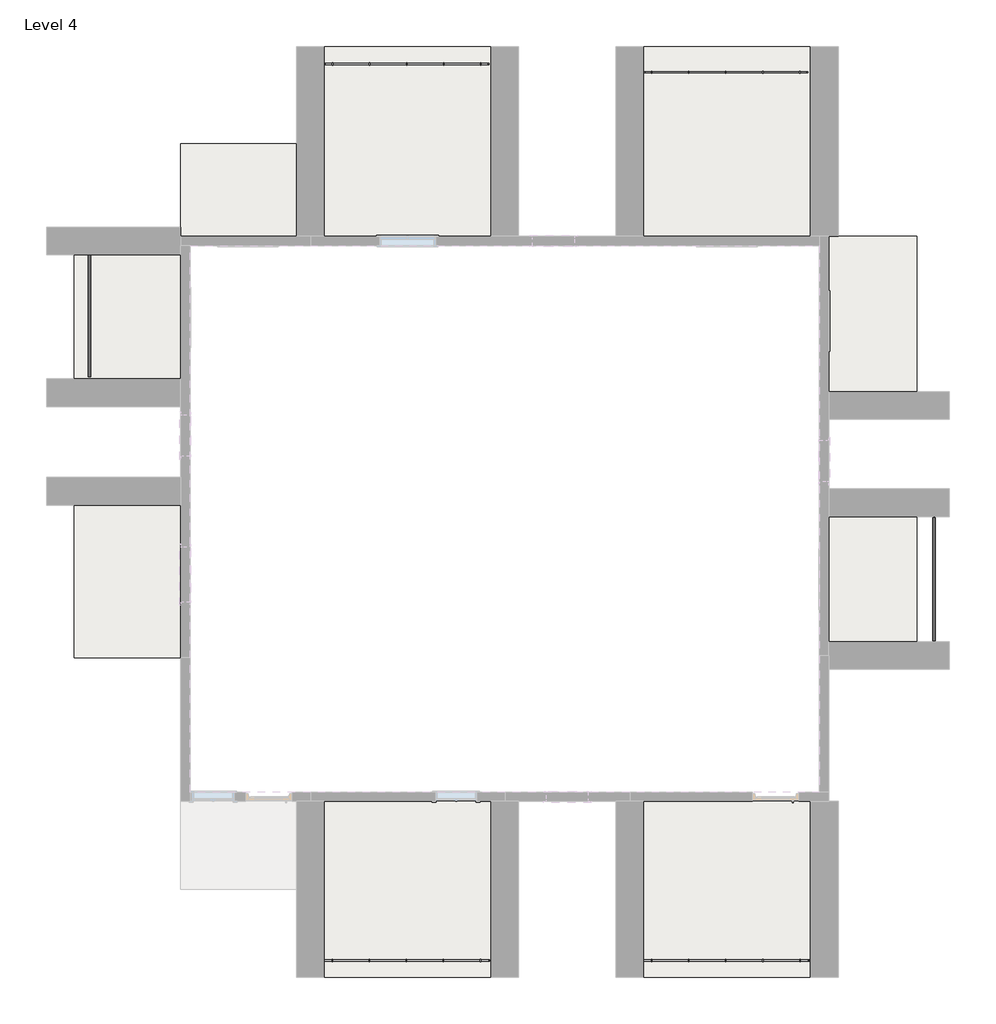
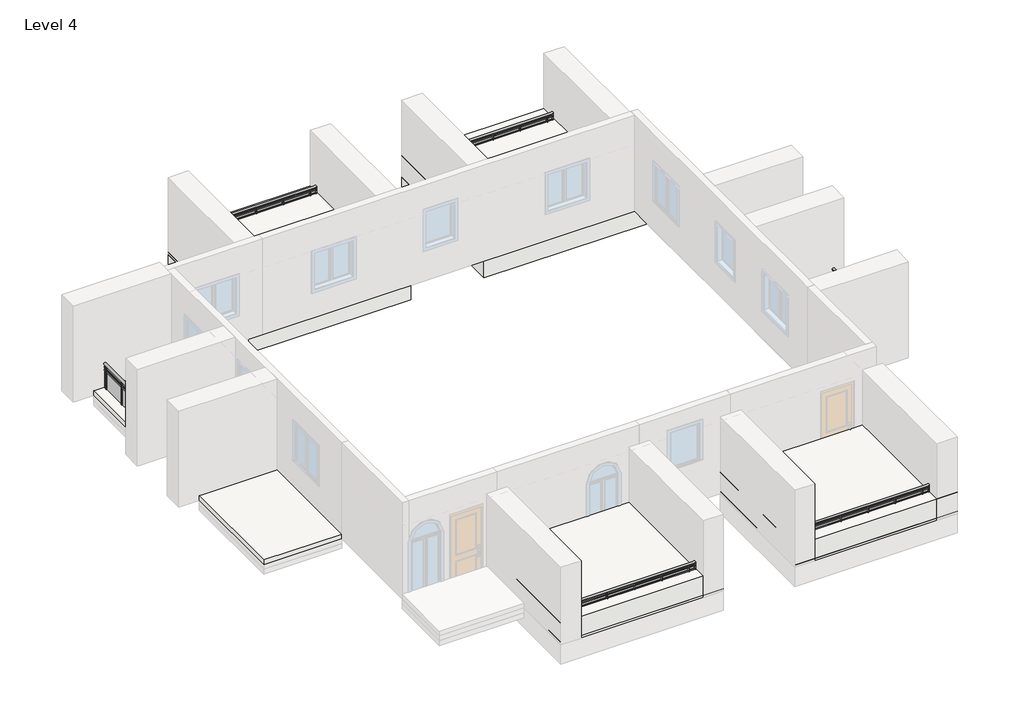
# One storey, part 2 of 2: 6 railings, 5 slabs.
"""IFC4 building model written with IfcOpenShell, lengths in millimetres."""

from ifc_helpers import new_model, si_unit, point, frame, origin, place, context, project, spatial, polyline, ellipse_curve, trimmed, outline, extrude, element, save
from ifc_brep_helpers import plane_surface, extruded_surface, advanced_brep

model = new_model("IFC4")

# Units and contexts
model_context = context("Model", 3, world=origin())
ifc_project = project(units=[si_unit("LENGTHUNIT", "METRE", prefix="MILLI")], contexts=[model_context])

# Site, building, storey
site = spatial("IfcSite", under=ifc_project)
building = spatial("IfcBuilding", under=site)
storey = spatial("IfcBuildingStorey", under=building, Name="Level 4", Elevation=9144.0)

# Railings
placement = place(None, origin())
element("IfcRailing", 1, ObjectType="Glass Panel - Bottom Fill", at=placement, inside=storey, context=model_context, shape_type="SolidModel", body=[
    advanced_brep(
    [(-9258.4937431, -9324.2034265, 10363.2), (-9258.4937431, -9400.4034265, 10363.2), (-5600.8937431, -9324.2034265, 10363.2), (-5600.8937431, -9400.4034265, 10363.2)],
    [
        (0, 1, ellipse_curve(frame((-9258.4937431, -9362.3034265, 10363.2), z_axis=(-1.0, 0.0, 0.0), x_axis=(0.0, -1.0, 0.0)), 38.1, 28.575)),
        (1, 0, ellipse_curve(frame((-9258.4937431, -9362.3034265, 10363.2), z_axis=(-1.0, 0.0, 0.0), x_axis=(0.0, -1.0, 0.0)), 38.1, 28.575)),
        (2, 3, ellipse_curve(frame((-5600.8937431, -9362.3034265, 10363.2), z_axis=(1.0, 0.0, 0.0), x_axis=(0.0, -1.0, 0.0)), 38.1, 28.575)),
        (3, 2, ellipse_curve(frame((-5600.8937431, -9362.3034265, 10363.2), z_axis=(1.0, 0.0, 0.0), x_axis=(0.0, -1.0, 0.0)), 38.1, 28.575)),
        (0, 2),
        (3, 1),
    ],
    [
        plane_surface(frame((-9258.4937431, -9362.3034265, 10363.2), z_axis=(-1.0, 0.0, 0.0), x_axis=(0.0, 1.0, 0.0))),
        plane_surface(frame((-5600.8937431, -9362.3034265, 10363.2), z_axis=(1.0, 0.0, 0.0), x_axis=(0.0, 1.0, 0.0))),
        extruded_surface(trimmed(ellipse_curve(frame((-5600.8937431, -9362.3034265, 10363.2), z_axis=(-1.0, 0.0, 0.0), x_axis=(0.0, -1.0, 0.0)), 38.1, 28.575), [point((-5600.8937431, -9324.2034265, 10363.2))], [point((-5600.8937431, -9400.4034265, 10363.2))], True, "CARTESIAN"), (-3657.5999999999995, 0.0, 0.0), 3657.5999999999995),
        extruded_surface(trimmed(ellipse_curve(frame((-5600.8937431, -9362.3034265, 10363.2), z_axis=(-1.0, 0.0, 0.0), x_axis=(0.0, -1.0, 0.0)), 38.1, 28.575), [point((-5600.8937431, -9400.4034265, 10363.2))], [point((-5600.8937431, -9324.2034265, 10363.2))], True, "CARTESIAN"), (-3657.5999999999995, 0.0, 0.0), 3657.5999999999995),
    ],
    [
        (0, [[1, 2]]),
        (1, [[3, 4]]),
        (2, [[-1, 5, -4, 6]]),
        (3, [[-2, -6, -3, -5]]),
    ],
),
    extrude(outline(polyline([(-9258.4937431, -9375.0034265), (-9258.4937431, -9349.6034265), (-5600.8937431, -9349.6034265), (-5600.8937431, -9375.0034265), (-9258.4937431, -9375.0034265)])), frame((0.0, 0.0, 10248.9), z_axis=(0.0, 0.0, 1.0), x_axis=(1.0, 0.0, 0.0)), (0.0, 0.0, 1.0), 25.4),
    extrude(outline(polyline([(-9258.4937431, -9375.0034265), (-9258.4937431, -9349.6034265), (-5600.8937431, -9349.6034265), (-5600.8937431, -9375.0034265), (-9258.4937431, -9375.0034265)])), frame((0.0, 0.0, 10147.3), z_axis=(0.0, 0.0, 1.0), x_axis=(1.0, 0.0, 0.0)), (0.0, 0.0, 1.0), 25.4),
    extrude(outline(polyline([(-5810.4437431, -9387.7034265), (-5810.4437431, -9336.9034265), (-5797.7437431, -9336.9034265), (-5797.7437431, -9387.7034265), (-5810.4437431, -9387.7034265)])), frame((0.0, 0.0, 9448.8), z_axis=(0.0, 0.0, 1.0), x_axis=(1.0, 0.0, 0.0)), (0.0, 0.0, 1.0), 885.6788223),
    extrude(outline(polyline([(-6616.8937431, -9355.7682695), (-5804.0937431, -9355.7682695), (-5804.0937431, -9362.1182695), (-6616.8937431, -9362.1182695), (-6616.8937431, -9355.7682695)])), frame((0.0, 0.0, 9550.4), z_axis=(0.0, 0.0, 1.0), x_axis=(1.0, 0.0, 0.0)), (0.0, 0.0, 1.0), 596.9),
    extrude(outline(polyline([(-6623.2437431, -9387.7034265), (-6623.2437431, -9336.9034265), (-6610.5437431, -9336.9034265), (-6610.5437431, -9387.7034265), (-6623.2437431, -9387.7034265)])), frame((0.0, 0.0, 9448.8), z_axis=(0.0, 0.0, 1.0), x_axis=(1.0, 0.0, 0.0)), (0.0, 0.0, 1.0), 885.6788223),
    extrude(outline(polyline([(-7429.6937431, -9355.7682695), (-6616.8937431, -9355.7682695), (-6616.8937431, -9362.1182695), (-7429.6937431, -9362.1182695), (-7429.6937431, -9355.7682695)])), frame((0.0, 0.0, 9550.4), z_axis=(0.0, 0.0, 1.0), x_axis=(1.0, 0.0, 0.0)), (0.0, 0.0, 1.0), 596.9),
    extrude(outline(polyline([(-7436.0437431, -9387.7034265), (-7436.0437431, -9336.9034265), (-7423.3437431, -9336.9034265), (-7423.3437431, -9387.7034265), (-7436.0437431, -9387.7034265)])), frame((0.0, 0.0, 9448.8), z_axis=(0.0, 0.0, 1.0), x_axis=(1.0, 0.0, 0.0)), (0.0, 0.0, 1.0), 885.6788223),
    extrude(outline(polyline([(-8242.4937431, -9355.7682695), (-7429.6937431, -9355.7682695), (-7429.6937431, -9362.1182695), (-8242.4937431, -9362.1182695), (-8242.4937431, -9355.7682695)])), frame((0.0, 0.0, 9550.4), z_axis=(0.0, 0.0, 1.0), x_axis=(1.0, 0.0, 0.0)), (0.0, 0.0, 1.0), 596.9),
    extrude(outline(polyline([(-8248.8437431, -9387.7034265), (-8248.8437431, -9336.9034265), (-8236.1437431, -9336.9034265), (-8236.1437431, -9387.7034265), (-8248.8437431, -9387.7034265)])), frame((0.0, 0.0, 9448.8), z_axis=(0.0, 0.0, 1.0), x_axis=(1.0, 0.0, 0.0)), (0.0, 0.0, 1.0), 885.6788223),
    extrude(outline(polyline([(-9055.2937431, -9355.7682695), (-8242.4937431, -9355.7682695), (-8242.4937431, -9362.1182695), (-9055.2937431, -9362.1182695), (-9055.2937431, -9355.7682695)])), frame((0.0, 0.0, 9550.4), z_axis=(0.0, 0.0, 1.0), x_axis=(1.0, 0.0, 0.0)), (0.0, 0.0, 1.0), 596.9),
    extrude(outline(polyline([(-9061.6437431, -9387.7034265), (-9061.6437431, -9336.9034265), (-9048.9437431, -9336.9034265), (-9048.9437431, -9387.7034265), (-9061.6437431, -9387.7034265)])), frame((0.0, 0.0, 9448.8), z_axis=(0.0, 0.0, 1.0), x_axis=(1.0, 0.0, 0.0)), (0.0, 0.0, 1.0), 885.6788223),
    extrude(outline(polyline([(-5613.5937431, -9371.8284265), (-5613.5937431, -9352.7784265), (-5594.5437431, -9352.7784265), (-5594.5437431, -9371.8284265), (-5613.5937431, -9371.8284265)])), frame((0.0, 0.0, 9448.8), z_axis=(0.0, 0.0, 1.0), x_axis=(1.0, 0.0, 0.0)), (0.0, 0.0, 1.0), 885.6788223),
    extrude(outline(polyline([(-9264.8437431, -9371.8284265), (-9264.8437431, -9352.7784265), (-9245.7937431, -9352.7784265), (-9245.7937431, -9371.8284265), (-9264.8437431, -9371.8284265)])), frame((0.0, 0.0, 9448.8), z_axis=(0.0, 0.0, 1.0), x_axis=(1.0, 0.0, 0.0)), (0.0, 0.0, 1.0), 885.6788223),
])
element("IfcRailing", 2, ObjectType="Glass Panel - Bottom Fill", at=placement, inside=storey, context=model_context, shape_type="SolidModel", body=[
    advanced_brep(
    [(-2248.0325613, -9324.2034265, 10358.1393423), (-2248.0325613, -9400.4034265, 10358.1393423), (1409.5674387, -9324.2034265, 10358.1393423), (1409.5674387, -9400.4034265, 10358.1393423)],
    [
        (0, 1, ellipse_curve(frame((-2248.0325613, -9362.3034265, 10358.1393423), z_axis=(-1.0, 0.0, 0.0), x_axis=(0.0, -1.0, 0.0)), 38.1, 28.575)),
        (1, 0, ellipse_curve(frame((-2248.0325613, -9362.3034265, 10358.1393423), z_axis=(-1.0, 0.0, 0.0), x_axis=(0.0, -1.0, 0.0)), 38.1, 28.575)),
        (2, 3, ellipse_curve(frame((1409.5674387, -9362.3034265, 10358.1393423), z_axis=(1.0, 0.0, 0.0), x_axis=(0.0, -1.0, 0.0)), 38.1, 28.575)),
        (3, 2, ellipse_curve(frame((1409.5674387, -9362.3034265, 10358.1393423), z_axis=(1.0, 0.0, 0.0), x_axis=(0.0, -1.0, 0.0)), 38.1, 28.575)),
        (0, 2),
        (3, 1),
    ],
    [
        plane_surface(frame((-2248.0325613, -9362.3034265, 10358.1393423), z_axis=(-1.0, 0.0, 0.0), x_axis=(0.0, 1.0, 0.0))),
        plane_surface(frame((1409.5674387, -9362.3034265, 10358.1393423), z_axis=(1.0, 0.0, 0.0), x_axis=(0.0, 1.0, 0.0))),
        extruded_surface(trimmed(ellipse_curve(frame((1409.5674387, -9362.3034265, 10358.1393423), z_axis=(-1.0, 0.0, 0.0), x_axis=(0.0, -1.0, 0.0)), 38.1, 28.575), [point((1409.5674387, -9324.2034265, 10358.1393423))], [point((1409.5674387, -9400.4034265, 10358.1393423))], True, "CARTESIAN"), (-3657.6, 0.0, 0.0), 3657.6),
        extruded_surface(trimmed(ellipse_curve(frame((1409.5674387, -9362.3034265, 10358.1393423), z_axis=(-1.0, 0.0, 0.0), x_axis=(0.0, -1.0, 0.0)), 38.1, 28.575), [point((1409.5674387, -9400.4034265, 10358.1393423))], [point((1409.5674387, -9324.2034265, 10358.1393423))], True, "CARTESIAN"), (-3657.6, 0.0, 0.0), 3657.6),
    ],
    [
        (0, [[1, 2]]),
        (1, [[3, 4]]),
        (2, [[-1, 5, -4, 6]]),
        (3, [[-2, -6, -3, -5]]),
    ],
),
    extrude(outline(polyline([(-2248.0325613, -9375.0034265), (-2248.0325613, -9349.6034265), (1409.5674387, -9349.6034265), (1409.5674387, -9375.0034265), (-2248.0325613, -9375.0034265)])), frame((0.0, 0.0, 10243.8393423), z_axis=(0.0, 0.0, 1.0), x_axis=(1.0, 0.0, 0.0)), (0.0, 0.0, 1.0), 25.4),
    extrude(outline(polyline([(-2248.0325613, -9375.0034265), (-2248.0325613, -9349.6034265), (1409.5674387, -9349.6034265), (1409.5674387, -9375.0034265), (-2248.0325613, -9375.0034265)])), frame((0.0, 0.0, 10142.2393423), z_axis=(0.0, 0.0, 1.0), x_axis=(1.0, 0.0, 0.0)), (0.0, 0.0, 1.0), 25.4),
    extrude(outline(polyline([(1200.0174387, -9387.7034265), (1200.0174387, -9336.9034265), (1212.7174387, -9336.9034265), (1212.7174387, -9387.7034265), (1200.0174387, -9387.7034265)])), frame((0.0, 0.0, 9443.7393423), z_axis=(0.0, 0.0, 1.0), x_axis=(1.0, 0.0, 0.0)), (0.0, 0.0, 1.0), 885.6788223),
    extrude(outline(polyline([(393.5674387, -9355.7682695), (1206.3674387, -9355.7682695), (1206.3674387, -9362.1182695), (393.5674387, -9362.1182695), (393.5674387, -9355.7682695)])), frame((0.0, 0.0, 9545.3393423), z_axis=(0.0, 0.0, 1.0), x_axis=(1.0, 0.0, 0.0)), (0.0, 0.0, 1.0), 596.9),
    extrude(outline(polyline([(387.2174387, -9387.7034265), (387.2174387, -9336.9034265), (399.9174387, -9336.9034265), (399.9174387, -9387.7034265), (387.2174387, -9387.7034265)])), frame((0.0, 0.0, 9443.7393423), z_axis=(0.0, 0.0, 1.0), x_axis=(1.0, 0.0, 0.0)), (0.0, 0.0, 1.0), 885.6788223),
    extrude(outline(polyline([(-419.2325613, -9355.7682695), (393.5674387, -9355.7682695), (393.5674387, -9362.1182695), (-419.2325613, -9362.1182695), (-419.2325613, -9355.7682695)])), frame((0.0, 0.0, 9545.3393423), z_axis=(0.0, 0.0, 1.0), x_axis=(1.0, 0.0, 0.0)), (0.0, 0.0, 1.0), 596.9),
    extrude(outline(polyline([(-425.5825613, -9387.7034265), (-425.5825613, -9336.9034265), (-412.8825613, -9336.9034265), (-412.8825613, -9387.7034265), (-425.5825613, -9387.7034265)])), frame((0.0, 0.0, 9443.7393423), z_axis=(0.0, 0.0, 1.0), x_axis=(1.0, 0.0, 0.0)), (0.0, 0.0, 1.0), 885.6788223),
    extrude(outline(polyline([(-1232.0325613, -9355.7682695), (-419.2325613, -9355.7682695), (-419.2325613, -9362.1182695), (-1232.0325613, -9362.1182695), (-1232.0325613, -9355.7682695)])), frame((0.0, 0.0, 9545.3393423), z_axis=(0.0, 0.0, 1.0), x_axis=(1.0, 0.0, 0.0)), (0.0, 0.0, 1.0), 596.9),
    extrude(outline(polyline([(-1238.3825613, -9387.7034265), (-1238.3825613, -9336.9034265), (-1225.6825613, -9336.9034265), (-1225.6825613, -9387.7034265), (-1238.3825613, -9387.7034265)])), frame((0.0, 0.0, 9443.7393423), z_axis=(0.0, 0.0, 1.0), x_axis=(1.0, 0.0, 0.0)), (0.0, 0.0, 1.0), 885.6788223),
    extrude(outline(polyline([(-2044.8325613, -9355.7682695), (-1232.0325613, -9355.7682695), (-1232.0325613, -9362.1182695), (-2044.8325613, -9362.1182695), (-2044.8325613, -9355.7682695)])), frame((0.0, 0.0, 9545.3393423), z_axis=(0.0, 0.0, 1.0), x_axis=(1.0, 0.0, 0.0)), (0.0, 0.0, 1.0), 596.9),
    extrude(outline(polyline([(-2051.1825613, -9387.7034265), (-2051.1825613, -9336.9034265), (-2038.4825613, -9336.9034265), (-2038.4825613, -9387.7034265), (-2051.1825613, -9387.7034265)])), frame((0.0, 0.0, 9443.7393423), z_axis=(0.0, 0.0, 1.0), x_axis=(1.0, 0.0, 0.0)), (0.0, 0.0, 1.0), 885.6788223),
    extrude(outline(polyline([(1396.8674387, -9371.8284265), (1396.8674387, -9352.7784265), (1415.9174387, -9352.7784265), (1415.9174387, -9371.8284265), (1396.8674387, -9371.8284265)])), frame((0.0, 0.0, 9443.7393423), z_axis=(0.0, 0.0, 1.0), x_axis=(1.0, 0.0, 0.0)), (0.0, 0.0, 1.0), 885.6788223),
    extrude(outline(polyline([(-2254.3825613, -9371.8284265), (-2254.3825613, -9352.7784265), (-2235.3325613, -9352.7784265), (-2235.3325613, -9371.8284265), (-2254.3825613, -9371.8284265)])), frame((0.0, 0.0, 9443.7393423), z_axis=(0.0, 0.0, 1.0), x_axis=(1.0, 0.0, 0.0)), (0.0, 0.0, 1.0), 885.6788223),
])
element("IfcRailing", 3, ObjectType="Glass Panel - Bottom Fill", at=placement, inside=storey, context=model_context, shape_type="SolidModel", body=[
    advanced_brep(
    [(-14351.1937431, 6115.813611, 10363.2), (-14427.3937431, 6115.813611, 10363.2), (-14351.1937431, 3448.813611, 10363.2), (-14427.3937431, 3448.813611, 10363.2)],
    [
        (0, 1, ellipse_curve(frame((-14389.2937431, 6115.813611, 10363.2), z_axis=(0.0, 1.0, 0.0), x_axis=(-1.0, 0.0, 0.0)), 38.1, 28.575)),
        (1, 0, ellipse_curve(frame((-14389.2937431, 6115.813611, 10363.2), z_axis=(0.0, 1.0, 0.0), x_axis=(-1.0, 0.0, 0.0)), 38.1, 28.575)),
        (2, 3, ellipse_curve(frame((-14389.2937431, 3448.813611, 10363.2), z_axis=(0.0, -1.0, 0.0), x_axis=(-1.0, 0.0, 0.0)), 38.1, 28.575)),
        (3, 2, ellipse_curve(frame((-14389.2937431, 3448.813611, 10363.2), z_axis=(0.0, -1.0, 0.0), x_axis=(-1.0, 0.0, 0.0)), 38.1, 28.575)),
        (0, 2),
        (3, 1),
    ],
    [
        plane_surface(frame((-14389.2937431, 6115.813611, 10363.2), z_axis=(0.0, 1.0, 0.0), x_axis=(0.0, 0.0, -1.0))),
        plane_surface(frame((-14389.2937431, 3448.813611, 10363.2), z_axis=(0.0, -1.0, 0.0), x_axis=(0.0, 0.0, -1.0))),
        extruded_surface(trimmed(ellipse_curve(frame((-14389.2937431, 3448.813611, 10363.2), z_axis=(0.0, 1.0, 0.0), x_axis=(-1.0, 0.0, 0.0)), 38.1, 28.575), [point((-14351.1937431, 3448.813611, 10363.2))], [point((-14427.3937431, 3448.813611, 10363.2))], True, "CARTESIAN"), (0.0, 2666.9999999999995, 0.0), 2666.9999999999995),
        extruded_surface(trimmed(ellipse_curve(frame((-14389.2937431, 3448.813611, 10363.2), z_axis=(0.0, 1.0, 0.0), x_axis=(-1.0, 0.0, 0.0)), 38.1, 28.575), [point((-14427.3937431, 3448.813611, 10363.2))], [point((-14351.1937431, 3448.813611, 10363.2))], True, "CARTESIAN"), (0.0, 2666.9999999999995, 0.0), 2666.9999999999995),
    ],
    [
        (0, [[1, 2]]),
        (1, [[3, 4]]),
        (2, [[-1, 5, -4, 6]]),
        (3, [[-2, -6, -3, -5]]),
    ],
),
    extrude(outline(polyline([(-14401.9937431, 6115.813611), (-14376.5937431, 6115.813611), (-14376.5937431, 3448.813611), (-14401.9937431, 3448.813611), (-14401.9937431, 6115.813611)])), frame((0.0, 0.0, 10248.9), z_axis=(0.0, 0.0, 1.0), x_axis=(1.0, 0.0, 0.0)), (0.0, 0.0, 1.0), 25.4),
    extrude(outline(polyline([(-14401.9937431, 6115.813611), (-14376.5937431, 6115.813611), (-14376.5937431, 3448.813611), (-14401.9937431, 3448.813611), (-14401.9937431, 6115.813611)])), frame((0.0, 0.0, 10147.3), z_axis=(0.0, 0.0, 1.0), x_axis=(1.0, 0.0, 0.0)), (0.0, 0.0, 1.0), 25.4),
    extrude(outline(polyline([(-14414.6937431, 3569.463611), (-14363.8937431, 3569.463611), (-14363.8937431, 3556.763611), (-14414.6937431, 3556.763611), (-14414.6937431, 3569.463611)])), frame((0.0, 0.0, 9448.8), z_axis=(0.0, 0.0, 1.0), x_axis=(1.0, 0.0, 0.0)), (0.0, 0.0, 1.0), 885.6788223),
    extrude(outline(polyline([(-14382.7585861, 4375.913611), (-14382.7585861, 3563.113611), (-14389.1085861, 3563.113611), (-14389.1085861, 4375.913611), (-14382.7585861, 4375.913611)])), frame((0.0, 0.0, 9550.4), z_axis=(0.0, 0.0, 1.0), x_axis=(1.0, 0.0, 0.0)), (0.0, 0.0, 1.0), 596.9),
    extrude(outline(polyline([(-14414.6937431, 4382.263611), (-14363.8937431, 4382.263611), (-14363.8937431, 4369.563611), (-14414.6937431, 4369.563611), (-14414.6937431, 4382.263611)])), frame((0.0, 0.0, 9448.8), z_axis=(0.0, 0.0, 1.0), x_axis=(1.0, 0.0, 0.0)), (0.0, 0.0, 1.0), 885.6788223),
    extrude(outline(polyline([(-14382.7585861, 5188.713611), (-14382.7585861, 4375.913611), (-14389.1085861, 4375.913611), (-14389.1085861, 5188.713611), (-14382.7585861, 5188.713611)])), frame((0.0, 0.0, 9550.4), z_axis=(0.0, 0.0, 1.0), x_axis=(1.0, 0.0, 0.0)), (0.0, 0.0, 1.0), 596.9),
    extrude(outline(polyline([(-14414.6937431, 5195.063611), (-14363.8937431, 5195.063611), (-14363.8937431, 5182.363611), (-14414.6937431, 5182.363611), (-14414.6937431, 5195.063611)])), frame((0.0, 0.0, 9448.8), z_axis=(0.0, 0.0, 1.0), x_axis=(1.0, 0.0, 0.0)), (0.0, 0.0, 1.0), 885.6788223),
    extrude(outline(polyline([(-14382.7585861, 6001.513611), (-14382.7585861, 5188.713611), (-14389.1085861, 5188.713611), (-14389.1085861, 6001.513611), (-14382.7585861, 6001.513611)])), frame((0.0, 0.0, 9550.4), z_axis=(0.0, 0.0, 1.0), x_axis=(1.0, 0.0, 0.0)), (0.0, 0.0, 1.0), 596.9),
    extrude(outline(polyline([(-14414.6937431, 6007.863611), (-14363.8937431, 6007.863611), (-14363.8937431, 5995.163611), (-14414.6937431, 5995.163611), (-14414.6937431, 6007.863611)])), frame((0.0, 0.0, 9448.8), z_axis=(0.0, 0.0, 1.0), x_axis=(1.0, 0.0, 0.0)), (0.0, 0.0, 1.0), 885.6788223),
    extrude(outline(polyline([(-14398.8187431, 3461.513611), (-14379.7687431, 3461.513611), (-14379.7687431, 3442.463611), (-14398.8187431, 3442.463611), (-14398.8187431, 3461.513611)])), frame((0.0, 0.0, 9448.8), z_axis=(0.0, 0.0, 1.0), x_axis=(1.0, 0.0, 0.0)), (0.0, 0.0, 1.0), 885.6788223),
    extrude(outline(polyline([(-14398.8187431, 6122.163611), (-14379.7687431, 6122.163611), (-14379.7687431, 6103.113611), (-14398.8187431, 6103.113611), (-14398.8187431, 6122.163611)])), frame((0.0, 0.0, 9448.8), z_axis=(0.0, 0.0, 1.0), x_axis=(1.0, 0.0, 0.0)), (0.0, 0.0, 1.0), 885.6788223),
])
element("IfcRailing", 4, ObjectType="Glass Panel - Bottom Fill", at=placement, inside=storey, context=model_context, shape_type="SolidModel", body=[
    advanced_brep(
    [(-9229.0758442, 10344.5205237, 10363.2), (-9229.0758442, 10268.3205237, 10363.2), (-5622.2758442, 10344.5205237, 10363.2), (-5622.2758442, 10268.3205237, 10363.2)],
    [
        (0, 1, ellipse_curve(frame((-9229.0758442, 10306.4205237, 10363.2), z_axis=(-1.0, 0.0, 0.0), x_axis=(0.0, -1.0, 0.0)), 38.1, 28.575)),
        (1, 0, ellipse_curve(frame((-9229.0758442, 10306.4205237, 10363.2), z_axis=(-1.0, 0.0, 0.0), x_axis=(0.0, -1.0, 0.0)), 38.1, 28.575)),
        (2, 3, ellipse_curve(frame((-5622.2758442, 10306.4205237, 10363.2), z_axis=(1.0, 0.0, 0.0), x_axis=(0.0, -1.0, 0.0)), 38.1, 28.575)),
        (3, 2, ellipse_curve(frame((-5622.2758442, 10306.4205237, 10363.2), z_axis=(1.0, 0.0, 0.0), x_axis=(0.0, -1.0, 0.0)), 38.1, 28.575)),
        (0, 2),
        (3, 1),
    ],
    [
        plane_surface(frame((-9229.0758442, 10306.4205237, 10363.2), z_axis=(-1.0, 0.0, 0.0), x_axis=(0.0, 1.0, 0.0))),
        plane_surface(frame((-5622.2758442, 10306.4205237, 10363.2), z_axis=(1.0, 0.0, 0.0), x_axis=(0.0, 1.0, 0.0))),
        extruded_surface(trimmed(ellipse_curve(frame((-5622.2758442, 10306.4205237, 10363.2), z_axis=(-1.0, 0.0, 0.0), x_axis=(0.0, -1.0, 0.0)), 38.1, 28.575), [point((-5622.2758442, 10344.5205237, 10363.2))], [point((-5622.2758442, 10268.3205237, 10363.2))], True, "CARTESIAN"), (-3606.8, 0.0, 0.0), 3606.8),
        extruded_surface(trimmed(ellipse_curve(frame((-5622.2758442, 10306.4205237, 10363.2), z_axis=(-1.0, 0.0, 0.0), x_axis=(0.0, -1.0, 0.0)), 38.1, 28.575), [point((-5622.2758442, 10268.3205237, 10363.2))], [point((-5622.2758442, 10344.5205237, 10363.2))], True, "CARTESIAN"), (-3606.8, 0.0, 0.0), 3606.8),
    ],
    [
        (0, [[1, 2]]),
        (1, [[3, 4]]),
        (2, [[-1, 5, -4, 6]]),
        (3, [[-2, -6, -3, -5]]),
    ],
),
    extrude(outline(polyline([(-9229.0758442, 10293.7205237), (-9229.0758442, 10319.1205237), (-5622.2758442, 10319.1205237), (-5622.2758442, 10293.7205237), (-9229.0758442, 10293.7205237)])), frame((0.0, 0.0, 10248.9), z_axis=(0.0, 0.0, 1.0), x_axis=(1.0, 0.0, 0.0)), (0.0, 0.0, 1.0), 25.4),
    extrude(outline(polyline([(-9229.0758442, 10293.7205237), (-9229.0758442, 10319.1205237), (-5622.2758442, 10319.1205237), (-5622.2758442, 10293.7205237), (-9229.0758442, 10293.7205237)])), frame((0.0, 0.0, 10147.3), z_axis=(0.0, 0.0, 1.0), x_axis=(1.0, 0.0, 0.0)), (0.0, 0.0, 1.0), 25.4),
    extrude(outline(polyline([(-5806.4258442, 10281.0205237), (-5806.4258442, 10331.8205237), (-5793.7258442, 10331.8205237), (-5793.7258442, 10281.0205237), (-5806.4258442, 10281.0205237)])), frame((0.0, 0.0, 9448.8), z_axis=(0.0, 0.0, 1.0), x_axis=(1.0, 0.0, 0.0)), (0.0, 0.0, 1.0), 885.6788223),
    extrude(outline(polyline([(-6612.8758442, 10312.9556807), (-5800.0758442, 10312.9556807), (-5800.0758442, 10306.6056807), (-6612.8758442, 10306.6056807), (-6612.8758442, 10312.9556807)])), frame((0.0, 0.0, 9550.4), z_axis=(0.0, 0.0, 1.0), x_axis=(1.0, 0.0, 0.0)), (0.0, 0.0, 1.0), 596.9),
    extrude(outline(polyline([(-6619.2258442, 10281.0205237), (-6619.2258442, 10331.8205237), (-6606.5258442, 10331.8205237), (-6606.5258442, 10281.0205237), (-6619.2258442, 10281.0205237)])), frame((0.0, 0.0, 9448.8), z_axis=(0.0, 0.0, 1.0), x_axis=(1.0, 0.0, 0.0)), (0.0, 0.0, 1.0), 885.6788223),
    extrude(outline(polyline([(-7425.6758442, 10312.9556807), (-6612.8758442, 10312.9556807), (-6612.8758442, 10306.6056807), (-7425.6758442, 10306.6056807), (-7425.6758442, 10312.9556807)])), frame((0.0, 0.0, 9550.4), z_axis=(0.0, 0.0, 1.0), x_axis=(1.0, 0.0, 0.0)), (0.0, 0.0, 1.0), 596.9),
    extrude(outline(polyline([(-7432.0258442, 10281.0205237), (-7432.0258442, 10331.8205237), (-7419.3258442, 10331.8205237), (-7419.3258442, 10281.0205237), (-7432.0258442, 10281.0205237)])), frame((0.0, 0.0, 9448.8), z_axis=(0.0, 0.0, 1.0), x_axis=(1.0, 0.0, 0.0)), (0.0, 0.0, 1.0), 885.6788223),
    extrude(outline(polyline([(-8238.4758442, 10312.9556807), (-7425.6758442, 10312.9556807), (-7425.6758442, 10306.6056807), (-8238.4758442, 10306.6056807), (-8238.4758442, 10312.9556807)])), frame((0.0, 0.0, 9550.4), z_axis=(0.0, 0.0, 1.0), x_axis=(1.0, 0.0, 0.0)), (0.0, 0.0, 1.0), 596.9),
    extrude(outline(polyline([(-8244.8258442, 10281.0205237), (-8244.8258442, 10331.8205237), (-8232.1258442, 10331.8205237), (-8232.1258442, 10281.0205237), (-8244.8258442, 10281.0205237)])), frame((0.0, 0.0, 9448.8), z_axis=(0.0, 0.0, 1.0), x_axis=(1.0, 0.0, 0.0)), (0.0, 0.0, 1.0), 885.6788223),
    extrude(outline(polyline([(-9051.2758442, 10312.9556807), (-8238.4758442, 10312.9556807), (-8238.4758442, 10306.6056807), (-9051.2758442, 10306.6056807), (-9051.2758442, 10312.9556807)])), frame((0.0, 0.0, 9550.4), z_axis=(0.0, 0.0, 1.0), x_axis=(1.0, 0.0, 0.0)), (0.0, 0.0, 1.0), 596.9),
    extrude(outline(polyline([(-9057.6258442, 10281.0205237), (-9057.6258442, 10331.8205237), (-9044.9258442, 10331.8205237), (-9044.9258442, 10281.0205237), (-9057.6258442, 10281.0205237)])), frame((0.0, 0.0, 9448.8), z_axis=(0.0, 0.0, 1.0), x_axis=(1.0, 0.0, 0.0)), (0.0, 0.0, 1.0), 885.6788223),
    extrude(outline(polyline([(-5634.9758442, 10296.8955237), (-5634.9758442, 10315.9455237), (-5615.9258442, 10315.9455237), (-5615.9258442, 10296.8955237), (-5634.9758442, 10296.8955237)])), frame((0.0, 0.0, 9448.8), z_axis=(0.0, 0.0, 1.0), x_axis=(1.0, 0.0, 0.0)), (0.0, 0.0, 1.0), 885.6788223),
    extrude(outline(polyline([(-9235.4258442, 10296.8955237), (-9235.4258442, 10315.9455237), (-9216.3758442, 10315.9455237), (-9216.3758442, 10296.8955237), (-9235.4258442, 10296.8955237)])), frame((0.0, 0.0, 9448.8), z_axis=(0.0, 0.0, 1.0), x_axis=(1.0, 0.0, 0.0)), (0.0, 0.0, 1.0), 885.6788223),
])
element("IfcRailing", 5, ObjectType="Glass Panel - Bottom Fill", at=placement, inside=storey, context=model_context, shape_type="SolidModel", body=[
    advanced_brep(
    [(-2210.3891352, 10161.3373193, 10363.2), (-2210.3891352, 10085.1373193, 10363.2), (1371.0108648, 10161.3373193, 10363.2), (1371.0108648, 10085.1373193, 10363.2)],
    [
        (0, 1, ellipse_curve(frame((-2210.3891352, 10123.2373193, 10363.2), z_axis=(-1.0, 0.0, 0.0), x_axis=(0.0, -1.0, 0.0)), 38.1, 28.575)),
        (1, 0, ellipse_curve(frame((-2210.3891352, 10123.2373193, 10363.2), z_axis=(-1.0, 0.0, 0.0), x_axis=(0.0, -1.0, 0.0)), 38.1, 28.575)),
        (2, 3, ellipse_curve(frame((1371.0108648, 10123.2373193, 10363.2), z_axis=(1.0, 0.0, 0.0), x_axis=(0.0, -1.0, 0.0)), 38.1, 28.575)),
        (3, 2, ellipse_curve(frame((1371.0108648, 10123.2373193, 10363.2), z_axis=(1.0, 0.0, 0.0), x_axis=(0.0, -1.0, 0.0)), 38.1, 28.575)),
        (0, 2),
        (3, 1),
    ],
    [
        plane_surface(frame((-2210.3891352, 10123.2373193, 10363.2), z_axis=(-1.0, 0.0, 0.0), x_axis=(0.0, 1.0, 0.0))),
        plane_surface(frame((1371.0108648, 10123.2373193, 10363.2), z_axis=(1.0, 0.0, 0.0), x_axis=(0.0, 1.0, 0.0))),
        extruded_surface(trimmed(ellipse_curve(frame((1371.0108648, 10123.2373193, 10363.2), z_axis=(-1.0, 0.0, 0.0), x_axis=(0.0, -1.0, 0.0)), 38.1, 28.575), [point((1371.0108648, 10161.3373193, 10363.2))], [point((1371.0108648, 10085.1373193, 10363.2))], True, "CARTESIAN"), (-3581.4, 0.0, 0.0), 3581.4),
        extruded_surface(trimmed(ellipse_curve(frame((1371.0108648, 10123.2373193, 10363.2), z_axis=(-1.0, 0.0, 0.0), x_axis=(0.0, -1.0, 0.0)), 38.1, 28.575), [point((1371.0108648, 10085.1373193, 10363.2))], [point((1371.0108648, 10161.3373193, 10363.2))], True, "CARTESIAN"), (-3581.4, 0.0, 0.0), 3581.4),
    ],
    [
        (0, [[1, 2]]),
        (1, [[3, 4]]),
        (2, [[-1, 5, -4, 6]]),
        (3, [[-2, -6, -3, -5]]),
    ],
),
    extrude(outline(polyline([(-2210.3891352, 10110.5373193), (-2210.3891352, 10135.9373193), (1371.0108648, 10135.9373193), (1371.0108648, 10110.5373193), (-2210.3891352, 10110.5373193)])), frame((0.0, 0.0, 10248.9), z_axis=(0.0, 0.0, 1.0), x_axis=(1.0, 0.0, 0.0)), (0.0, 0.0, 1.0), 25.4),
    extrude(outline(polyline([(-2210.3891352, 10110.5373193), (-2210.3891352, 10135.9373193), (1371.0108648, 10135.9373193), (1371.0108648, 10110.5373193), (-2210.3891352, 10110.5373193)])), frame((0.0, 0.0, 10147.3), z_axis=(0.0, 0.0, 1.0), x_axis=(1.0, 0.0, 0.0)), (0.0, 0.0, 1.0), 25.4),
    extrude(outline(polyline([(1199.5608648, 10097.8373193), (1199.5608648, 10148.6373193), (1212.2608648, 10148.6373193), (1212.2608648, 10097.8373193), (1199.5608648, 10097.8373193)])), frame((0.0, 0.0, 9448.8), z_axis=(0.0, 0.0, 1.0), x_axis=(1.0, 0.0, 0.0)), (0.0, 0.0, 1.0), 885.6788223),
    extrude(outline(polyline([(393.1108648, 10129.7724763), (1205.9108648, 10129.7724763), (1205.9108648, 10123.4224763), (393.1108648, 10123.4224763), (393.1108648, 10129.7724763)])), frame((0.0, 0.0, 9550.4), z_axis=(0.0, 0.0, 1.0), x_axis=(1.0, 0.0, 0.0)), (0.0, 0.0, 1.0), 596.9),
    extrude(outline(polyline([(386.7608648, 10097.8373193), (386.7608648, 10148.6373193), (399.4608648, 10148.6373193), (399.4608648, 10097.8373193), (386.7608648, 10097.8373193)])), frame((0.0, 0.0, 9448.8), z_axis=(0.0, 0.0, 1.0), x_axis=(1.0, 0.0, 0.0)), (0.0, 0.0, 1.0), 885.6788223),
    extrude(outline(polyline([(-419.6891352, 10129.7724763), (393.1108648, 10129.7724763), (393.1108648, 10123.4224763), (-419.6891352, 10123.4224763), (-419.6891352, 10129.7724763)])), frame((0.0, 0.0, 9550.4), z_axis=(0.0, 0.0, 1.0), x_axis=(1.0, 0.0, 0.0)), (0.0, 0.0, 1.0), 596.9),
    extrude(outline(polyline([(-426.0391352, 10097.8373193), (-426.0391352, 10148.6373193), (-413.3391352, 10148.6373193), (-413.3391352, 10097.8373193), (-426.0391352, 10097.8373193)])), frame((0.0, 0.0, 9448.8), z_axis=(0.0, 0.0, 1.0), x_axis=(1.0, 0.0, 0.0)), (0.0, 0.0, 1.0), 885.6788223),
    extrude(outline(polyline([(-1232.4891352, 10129.7724763), (-419.6891352, 10129.7724763), (-419.6891352, 10123.4224763), (-1232.4891352, 10123.4224763), (-1232.4891352, 10129.7724763)])), frame((0.0, 0.0, 9550.4), z_axis=(0.0, 0.0, 1.0), x_axis=(1.0, 0.0, 0.0)), (0.0, 0.0, 1.0), 596.9),
    extrude(outline(polyline([(-1238.8391352, 10097.8373193), (-1238.8391352, 10148.6373193), (-1226.1391352, 10148.6373193), (-1226.1391352, 10097.8373193), (-1238.8391352, 10097.8373193)])), frame((0.0, 0.0, 9448.8), z_axis=(0.0, 0.0, 1.0), x_axis=(1.0, 0.0, 0.0)), (0.0, 0.0, 1.0), 885.6788223),
    extrude(outline(polyline([(-2045.2891352, 10129.7724763), (-1232.4891352, 10129.7724763), (-1232.4891352, 10123.4224763), (-2045.2891352, 10123.4224763), (-2045.2891352, 10129.7724763)])), frame((0.0, 0.0, 9550.4), z_axis=(0.0, 0.0, 1.0), x_axis=(1.0, 0.0, 0.0)), (0.0, 0.0, 1.0), 596.9),
    extrude(outline(polyline([(-2051.6391352, 10097.8373193), (-2051.6391352, 10148.6373193), (-2038.9391352, 10148.6373193), (-2038.9391352, 10097.8373193), (-2051.6391352, 10097.8373193)])), frame((0.0, 0.0, 9448.8), z_axis=(0.0, 0.0, 1.0), x_axis=(1.0, 0.0, 0.0)), (0.0, 0.0, 1.0), 885.6788223),
    extrude(outline(polyline([(1358.3108648, 10113.7123193), (1358.3108648, 10132.7623193), (1377.3608648, 10132.7623193), (1377.3608648, 10113.7123193), (1358.3108648, 10113.7123193)])), frame((0.0, 0.0, 9448.8), z_axis=(0.0, 0.0, 1.0), x_axis=(1.0, 0.0, 0.0)), (0.0, 0.0, 1.0), 885.6788223),
    extrude(outline(polyline([(-2216.7391352, 10113.7123193), (-2216.7391352, 10132.7623193), (-2197.6891352, 10132.7623193), (-2197.6891352, 10113.7123193), (-2216.7391352, 10113.7123193)])), frame((0.0, 0.0, 9448.8), z_axis=(0.0, 0.0, 1.0), x_axis=(1.0, 0.0, 0.0)), (0.0, 0.0, 1.0), 885.6788223),
])
element("IfcRailing", 6, ObjectType="Glass Panel - Bottom Fill", at=placement, inside=storey, context=model_context, shape_type="SolidModel", body=[
    advanced_brep(
    [(4190.8062569, 350.013611, 10363.2), (4114.6062569, 350.013611, 10363.2), (4190.8062569, -2342.386389, 10363.2), (4114.6062569, -2342.386389, 10363.2)],
    [
        (0, 1, ellipse_curve(frame((4152.7062569, 350.013611, 10363.2), z_axis=(0.0, 1.0, 0.0), x_axis=(-1.0, 0.0, 0.0)), 38.1, 28.575)),
        (1, 0, ellipse_curve(frame((4152.7062569, 350.013611, 10363.2), z_axis=(0.0, 1.0, 0.0), x_axis=(-1.0, 0.0, 0.0)), 38.1, 28.575)),
        (2, 3, ellipse_curve(frame((4152.7062569, -2342.386389, 10363.2), z_axis=(0.0, -1.0, 0.0), x_axis=(-1.0, 0.0, 0.0)), 38.1, 28.575)),
        (3, 2, ellipse_curve(frame((4152.7062569, -2342.386389, 10363.2), z_axis=(0.0, -1.0, 0.0), x_axis=(-1.0, 0.0, 0.0)), 38.1, 28.575)),
        (0, 2),
        (3, 1),
    ],
    [
        plane_surface(frame((4152.7062569, 350.013611, 10363.2), z_axis=(0.0, 1.0, 0.0), x_axis=(0.0, 0.0, -1.0))),
        plane_surface(frame((4152.7062569, -2342.386389, 10363.2), z_axis=(0.0, -1.0, 0.0), x_axis=(0.0, 0.0, -1.0))),
        extruded_surface(trimmed(ellipse_curve(frame((4152.7062569, -2342.386389, 10363.2), z_axis=(0.0, 1.0, 0.0), x_axis=(-1.0, 0.0, 0.0)), 38.1, 28.575), [point((4190.8062569, -2342.386389, 10363.2))], [point((4114.6062569, -2342.386389, 10363.2))], True, "CARTESIAN"), (0.0, 2692.3999999999996, 0.0), 2692.3999999999996),
        extruded_surface(trimmed(ellipse_curve(frame((4152.7062569, -2342.386389, 10363.2), z_axis=(0.0, 1.0, 0.0), x_axis=(-1.0, 0.0, 0.0)), 38.1, 28.575), [point((4114.6062569, -2342.386389, 10363.2))], [point((4190.8062569, -2342.386389, 10363.2))], True, "CARTESIAN"), (0.0, 2692.3999999999996, 0.0), 2692.3999999999996),
    ],
    [
        (0, [[1, 2]]),
        (1, [[3, 4]]),
        (2, [[-1, 5, -4, 6]]),
        (3, [[-2, -6, -3, -5]]),
    ],
),
    extrude(outline(polyline([(4140.0062569, 350.013611), (4165.4062569, 350.013611), (4165.4062569, -2342.386389), (4140.0062569, -2342.386389), (4140.0062569, 350.013611)])), frame((0.0, 0.0, 10248.9), z_axis=(0.0, 0.0, 1.0), x_axis=(1.0, 0.0, 0.0)), (0.0, 0.0, 1.0), 25.4),
    extrude(outline(polyline([(4140.0062569, 350.013611), (4165.4062569, 350.013611), (4165.4062569, -2342.386389), (4140.0062569, -2342.386389), (4140.0062569, 350.013611)])), frame((0.0, 0.0, 10147.3), z_axis=(0.0, 0.0, 1.0), x_axis=(1.0, 0.0, 0.0)), (0.0, 0.0, 1.0), 25.4),
    extrude(outline(polyline([(4127.3062569, -2209.036389), (4178.1062569, -2209.036389), (4178.1062569, -2221.736389), (4127.3062569, -2221.736389), (4127.3062569, -2209.036389)])), frame((0.0, 0.0, 9448.8), z_axis=(0.0, 0.0, 1.0), x_axis=(1.0, 0.0, 0.0)), (0.0, 0.0, 1.0), 885.6788223),
    extrude(outline(polyline([(4159.2414139, -1402.586389), (4159.2414139, -2215.386389), (4152.8914139, -2215.386389), (4152.8914139, -1402.586389), (4159.2414139, -1402.586389)])), frame((0.0, 0.0, 9550.4), z_axis=(0.0, 0.0, 1.0), x_axis=(1.0, 0.0, 0.0)), (0.0, 0.0, 1.0), 596.9),
    extrude(outline(polyline([(4127.3062569, -1396.236389), (4178.1062569, -1396.236389), (4178.1062569, -1408.936389), (4127.3062569, -1408.936389), (4127.3062569, -1396.236389)])), frame((0.0, 0.0, 9448.8), z_axis=(0.0, 0.0, 1.0), x_axis=(1.0, 0.0, 0.0)), (0.0, 0.0, 1.0), 885.6788223),
    extrude(outline(polyline([(4159.2414139, -589.786389), (4159.2414139, -1402.586389), (4152.8914139, -1402.586389), (4152.8914139, -589.786389), (4159.2414139, -589.786389)])), frame((0.0, 0.0, 9550.4), z_axis=(0.0, 0.0, 1.0), x_axis=(1.0, 0.0, 0.0)), (0.0, 0.0, 1.0), 596.9),
    extrude(outline(polyline([(4127.3062569, -583.436389), (4178.1062569, -583.436389), (4178.1062569, -596.136389), (4127.3062569, -596.136389), (4127.3062569, -583.436389)])), frame((0.0, 0.0, 9448.8), z_axis=(0.0, 0.0, 1.0), x_axis=(1.0, 0.0, 0.0)), (0.0, 0.0, 1.0), 885.6788223),
    extrude(outline(polyline([(4159.2414139, 223.013611), (4159.2414139, -589.786389), (4152.8914139, -589.786389), (4152.8914139, 223.013611), (4159.2414139, 223.013611)])), frame((0.0, 0.0, 9550.4), z_axis=(0.0, 0.0, 1.0), x_axis=(1.0, 0.0, 0.0)), (0.0, 0.0, 1.0), 596.9),
    extrude(outline(polyline([(4127.3062569, 229.363611), (4178.1062569, 229.363611), (4178.1062569, 216.663611), (4127.3062569, 216.663611), (4127.3062569, 229.363611)])), frame((0.0, 0.0, 9448.8), z_axis=(0.0, 0.0, 1.0), x_axis=(1.0, 0.0, 0.0)), (0.0, 0.0, 1.0), 885.6788223),
    extrude(outline(polyline([(4143.1812569, -2329.686389), (4162.2312569, -2329.686389), (4162.2312569, -2348.736389), (4143.1812569, -2348.736389), (4143.1812569, -2329.686389)])), frame((0.0, 0.0, 9448.8), z_axis=(0.0, 0.0, 1.0), x_axis=(1.0, 0.0, 0.0)), (0.0, 0.0, 1.0), 885.6788223),
    extrude(outline(polyline([(4143.1812569, 356.363611), (4162.2312569, 356.363611), (4162.2312569, 337.313611), (4143.1812569, 337.313611), (4143.1812569, 356.363611)])), frame((0.0, 0.0, 9448.8), z_axis=(0.0, 0.0, 1.0), x_axis=(1.0, 0.0, 0.0)), (0.0, 0.0, 1.0), 885.6788223),
])

# Slabs
element("IfcSlab", 7, ObjectType="Generic - 2'", at=placement, inside=storey, context=model_context, shape_type="SweptSolid", body=[
    extrude(outline(polyline([(-4965.8937431, 10687.813611), (-4965.8937431, 6522.213611), (-9842.6937431, 6522.213611), (-9842.6937431, 10687.813611), (-4965.8937431, 10687.813611)])), frame((0.0, 0.0, 8839.2), z_axis=(0.0, 0.0, 1.0), x_axis=(1.0, 0.0, 0.0)), (0.0, 0.0, 1.0), 609.6),
])
element("IfcSlab", 8, ObjectType="Generic - 2' 2", at=placement, inside=storey, context=model_context, shape_type="SweptSolid", body=[
    extrude(outline(polyline([(2044.5062569, 10687.813611), (2044.5062569, 6420.613611), (-2832.2937431, 6420.613611), (-2832.2937431, 10687.813611), (2044.5062569, 10687.813611)])), frame((0.0, 0.0, 8839.2), z_axis=(0.0, 0.0, 1.0), x_axis=(1.0, 0.0, 0.0)), (0.0, 0.0, 1.0), 609.6),
])
element("IfcSlab", 9, ObjectType="Generic - 2' 3", at=placement, inside=storey, context=model_context, shape_type="SweptSolid", body=[
    extrude(outline(polyline([(-4965.8937431, 6522.213611), (-9842.6937431, 6522.213611), (-9842.6937431, 10687.813611), (-4965.8937431, 10687.813611), (-4965.8937431, 6522.213611)])), frame((0.0, 0.0, 9448.8), z_axis=(0.0, 0.0, 1.0), x_axis=(1.0, 0.0, 0.0)), (0.0, 0.0, 1.0), 76.2),
    extrude(outline(polyline([(2044.5062569, 6522.213611), (-2832.2937431, 6522.213611), (-2832.2937431, 10687.813611), (2044.5062569, 10687.813611), (2044.5062569, 6522.213611)])), frame((0.0, 0.0, 9448.8), z_axis=(0.0, 0.0, 1.0), x_axis=(1.0, 0.0, 0.0)), (0.0, 0.0, 1.0), 76.2),
    extrude(outline(polyline([(-4965.8937431, -5872.986389), (-4965.8937431, -9733.786389), (-9842.6937431, -9733.786389), (-9842.6937431, -5872.986389), (-4965.8937431, -5872.986389)])), frame((0.0, 0.0, 9448.8), z_axis=(0.0, 0.0, 1.0), x_axis=(1.0, 0.0, 0.0)), (0.0, 0.0, 1.0), 76.2),
    extrude(outline(polyline([(2044.5062569, -5872.986389), (2044.5062569, -9733.786389), (-2832.2937431, -9733.786389), (-2832.2937431, -5872.986389), (2044.5062569, -5872.986389)])), frame((0.0, 0.0, 9448.8), z_axis=(0.0, 0.0, 1.0), x_axis=(1.0, 0.0, 0.0)), (0.0, 0.0, 1.0), 76.2),
])
element("IfcSlab", 10, ObjectType="Generic - 2' 4", at=placement, inside=storey, context=model_context, shape_type="SweptSolid", body=[
    extrude(outline(polyline([(-4965.8937431, 6522.213611), (-9842.6937431, 6522.213611), (-9842.6937431, 10687.813611), (-4965.8937431, 10687.813611), (-4965.8937431, 6522.213611)])), frame((0.0, 0.0, 9525.0), z_axis=(0.0, 0.0, 1.0), x_axis=(1.0, 0.0, 0.0)), (0.0, 0.0, 1.0), 609.6),
    extrude(outline(polyline([(2044.5062569, 6522.213611), (-2832.2937431, 6522.213611), (-2832.2937431, 10687.813611), (2044.5062569, 10687.813611), (2044.5062569, 6522.213611)])), frame((0.0, 0.0, 9525.0), z_axis=(0.0, 0.0, 1.0), x_axis=(1.0, 0.0, 0.0)), (0.0, 0.0, 1.0), 609.6),
    extrude(outline(polyline([(2044.5062569, -5872.986389), (2044.5062569, -9733.786389), (-2832.2937431, -9733.786389), (-2832.2937431, -5872.986389), (2044.5062569, -5872.986389)])), frame((0.0, 0.0, 9525.0), z_axis=(0.0, 0.0, 1.0), x_axis=(1.0, 0.0, 0.0)), (0.0, 0.0, 1.0), 609.6),
    extrude(outline(polyline([(-4965.8937431, -5872.986389), (-4965.8937431, -9733.786389), (-9842.6937431, -9733.786389), (-9842.6937431, -5872.986389), (-4965.8937431, -5872.986389)])), frame((0.0, 0.0, 9525.0), z_axis=(0.0, 0.0, 1.0), x_axis=(1.0, 0.0, 0.0)), (0.0, 0.0, 1.0), 609.6),
])
element("IfcSlab", 11, ObjectType="general 6\" 3", at=placement, inside=storey, context=model_context, shape_type="SweptSolid", body=[
    extrude(outline(polyline([(3771.7062569, 3118.613611), (1841.3062569, 3118.613611), (1841.3062569, 6522.213611), (3771.7062569, 6522.213611), (3771.7062569, 3118.613611)])), frame((0.0, 0.0, 9448.8), z_axis=(0.0, 0.0, 1.0), x_axis=(1.0, 0.0, 0.0)), (0.0, 0.0, 1.0), 152.4),
    extrude(outline(polyline([(3771.7062569, -2367.786389), (1841.3062569, -2367.786389), (1841.3062569, 375.413611), (3771.7062569, 375.413611), (3771.7062569, -2367.786389)])), frame((0.0, 0.0, 9448.8), z_axis=(0.0, 0.0, 1.0), x_axis=(1.0, 0.0, 0.0)), (0.0, 0.0, 1.0), 152.4),
    extrude(outline(polyline([(-12382.6937431, 6522.213611), (-12382.6937431, 8557.6995084), (-9842.6937431, 8557.6995084), (-9842.6937431, 6522.213611), (-12382.6937431, 6522.213611)])), frame((0.0, 0.0, 9448.8), z_axis=(0.0, 0.0, 1.0), x_axis=(1.0, 0.0, 0.0)), (0.0, 0.0, 1.0), 152.4),
    extrude(outline(polyline([(-14722.8064179, 3398.013611), (-14722.8064179, 6115.813611), (-12384.3500805, 6115.813611), (-12384.3500805, 3398.013611), (-14722.8064179, 3398.013611)])), frame((0.0, 0.0, 9448.8), z_axis=(0.0, 0.0, 1.0), x_axis=(1.0, 0.0, 0.0)), (0.0, 0.0, 1.0), 152.4),
    extrude(outline(polyline([(-14722.8064179, -2723.386389), (-14722.8064179, 629.413611), (-12382.6937431, 629.413611), (-12382.6937431, -2723.386389), (-14722.8064179, -2723.386389)])), frame((0.0, 0.0, 9448.8), z_axis=(0.0, 0.0, 1.0), x_axis=(1.0, 0.0, 0.0)), (0.0, 0.0, 1.0), 152.4),
])

save(model, "model.ifc")

# Revit data of these elements
# Type "Glass Panel - Bottom Fill"
#   Assembly Code = "C2010400"
#   built-in parameter 1008612 = 0.0416667 (stored number, unit not read)
#   built-in parameter 1008611 = 0.0416667 (stored number, unit not read)
#   built-in parameter 1008609 = 0.333333 (stored number, unit not read)
#   built-in parameter 1008604 = 0.166667 (stored number, unit not read)
#   built-in parameter 1008603 = 0.166667 (stored number, unit not read)
#   Railing Height = 3' - 0"
#   built-in parameter 1008630 = 2
#   built-in parameter 1008610 = 2
#   built-in parameter 1008618 = Baluster - Square : 3/4"
# Type "Generic - 2'"
#   Assembly Code = "B1010"
#   Function = 0
#   Layers, outside or top first: 2' - 0" no material (function 1)
# Type "Generic - 2' 2"
#   Assembly Code = "B1010"
#   Function = 0
#   Layers, outside or top first: 2' - 0" "Damp-proofing" (function 1)
# Type "Generic - 2' 3"
#   Assembly Code = "B1010"
#   Function = 0
#   Layers, outside or top first: 0' - 3" "Damp-proofing" (function 1)
# Type "Generic - 2' 4"
#   Assembly Code = "B1010"
#   Function = 0
#   Layers, outside or top first: 2' - 0" "Metal - Paint Finish - Grey" (function 1)
# Type "general 6\" 3"
#   Assembly Code = "B1010"
#   Function = 0
#   Layers, outside or top first: 0' - 6" "Door - Frame" (function 1)
# Elements 1, 3, 4, 5, 6 (IfcRailing, "Glass Panel - Bottom Fill")
#   built-in parameter 1008621 = 1 (stored number, unit not read)
#   Phase Created = New Construction
#   Materials on its faces: "Glass"
# Element 2 (IfcRailing, "Glass Panel - Bottom Fill")
#   built-in parameter 1008621 = 0.983397 (stored number, unit not read)
#   Phase Created = New Construction
#   Materials on its faces: "Glass"
# Element 7 (IfcSlab, "Generic - 2'")
#   Height Offset From Level = 1' - 0"
#   Phase Created = New Construction
#   Materials on its faces: "Default Floor", "Gypsum Wall Board"
# Element 8 (IfcSlab, "Generic - 2' 2")
#   Height Offset From Level = 1' - 0"
#   Phase Created = New Construction
#   Materials on its faces: "Gypsum Wall Board", "Damp-proofing"
# Element 9 (IfcSlab, "Generic - 2' 3")
#   Height Offset From Level = 1' - 3"
#   Phase Created = New Construction
#   Materials on its faces: "Damp-proofing"
# Element 10 (IfcSlab, "Generic - 2' 4")
#   Height Offset From Level = 3' - 3"
#   Phase Created = New Construction
#   Materials on its faces: "Metal - Paint Finish - Grey"
# Element 11 (IfcSlab, "general 6\" 3")
#   Height Offset From Level = 1' - 6"
#   Phase Created = New Construction
#   Materials on its faces: "Door - Frame"
# Materials
#   "Damp-proofing": class "Generic", colour RGB 127 127 127, transparency 0, Description = "Damp-proofing", Cost = 0
#   "Metal - Paint Finish - Grey": class "Paint", colour RGB 255 255 255, transparency 0, Cost = 0
#   "Door - Frame": colour RGB 118 70 51, transparency 0, Cost = 0
#   "Glass": class "Glass", colour RGB 0 128 192, transparency 0.75, Description = "Soda Lime Glass", Cost = 0
#   "Default Floor": colour RGB 128 128 128, transparency 0
#   "Gypsum Wall Board": class "Generic", colour RGB 127 127 127, transparency 0, Description = "Gypsum Wall Board", Cost = 0
